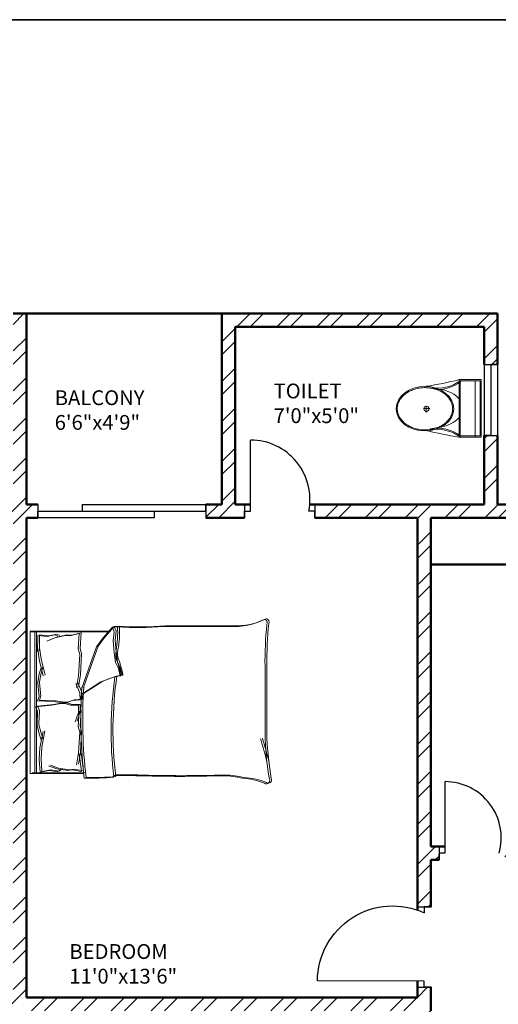
# Model space of a CAD drawing. Units: inches. Extents: x 963 to 2075, y 289 to 2657.
# Tile 95 of 98: x 1511 to 1672, y 2325 to 2657. Entities that reach past the tile are written whole.
import ezdxf

# ---------------------------------------------------------------- set-up
doc = ezdxf.new("R2010")
doc.units = ezdxf.units.IN
for name, color, linetype, lineweight in [('A-ANNO-TTLB', 7, 'Continuous', 35), ('A-AREA-IDEN', 7, 'Continuous', 18), ('A-DOOR', 4, 'Continuous', 25), ('A-FLOR-FIXT', 9, 'Continuous', 18), ('A-FURN', 8, 'Continuous', 18), ('A-GLAZ', 3, 'Continuous', 25), ('A-WALL', 7, 'Continuous', 50), ('A-WALL-PATT', 8, 'Continuous', 13)]:
    doc.layers.add(name, color=color, linetype=linetype, lineweight=lineweight)
doc.styles.get("Standard").update_dxf_attribs({"font": 'arial.ttf'})

# ---------------------------------------------------------------- blocks, each defined once
blk = doc.blocks.new('A$C31115884')
for p, q in [((283.1, 497.7), (223.4, 497.7)), ((257.5, 466.4), (257.5, 523.2)), ((0, 200), (0, 0)), ((520, 200), (0, 200)), ((10, 190), (10, 10)), ((510, 190), (10, 190)), ((510, 10), (510, 190)), ((520, 0), (520, 200)), ((510, 54.5), (0, 54.5)), ((10, 10), (510, 10)), ((0, 0), (520, 0))]:
    blk.add_line(p, q)
blk.add_circle((255.6, 496.4), 23.6)
for centre, radius, start, end in [((2777.7, -204.6), 2807, 165.4549, 171.71327), ((-294.5, 403.3), 364.7, 324.20913, 9.34987), ((-294.5, 403.3), 374.7, 324.20913, 9.34987), ((805.8, 403.3), 364.7, 170.65013, 215.79087), ((3237, 905), 2807, 188.28673, 194.5451), ((139.5, 406.2), 293.5, 315.84364, 2.65635), ((805.8, 403.3), 374.7, 179.20365, 215.79087), ((383.6, 406.2), 293.5, 190.27735, 224.15636)]:
    blk.add_arc(centre, radius, start, end)
blk.add_ellipse((256.2, 509.9), major_axis=(0, -260.7), ratio=0.772727)
blk.add_open_spline([(256.2, 259.2), (263.1, 259.2), (270, 259.7), (287.8, 262.3), (298.7, 265.1), (319.9, 273.1), (330.2, 278.4), (350.1, 291.1), (359.7, 298.7), (377.7, 315.9), (386.2, 325.5), (401.7, 346.6), (408.8, 358.1), (421.3, 382.5), (426.8, 395.5), (435.9, 422.4), (439.5, 436.4), (444.8, 465.1), (446.5, 479.7), (447.9, 509.2), (447.6, 524), (445, 553.3), (442.7, 567.8), (436.3, 596), (432.1, 609.7), (421.9, 636), (416, 648.6), (402.5, 672.1), (395, 683), (378.6, 703), (369.8, 712.1), (351.1, 728), (341.3, 734.8), (320.9, 746.2), (310.4, 750.7), (288.9, 757.3), (278, 759.4), (256, 761), (245, 760.6), (223.1, 757.2), (212.3, 754.3), (191.1, 746.1), (180.8, 740.7), (160.9, 727.8), (151.4, 720.1), (133.5, 702.7), (125.1, 693), (109.6, 671.7), (102.6, 660.2), (90.2, 635.7), (84.9, 622.7), (76, 595.6), (72.4, 581.6), (67.2, 552.9), (65.6, 538.2), (64.4, 508.8), (64.8, 494), (67.5, 464.7), (69.9, 450.2), (76.6, 422), (80.8, 408.3), (91.1, 382.2), (97.2, 369.7), (110.8, 346.3), (118.4, 335.4), (134.8, 315.6), (143.7, 306.7), (162.4, 290.9), (172.3, 284.2), (192.8, 273), (203.3, 268.6), (224.8, 262.2), (235.8, 260.2), (249.9, 259.3), (253, 259.2), (256.2, 259.2)], degree=3, knots=[0, 0, 0, 0, 0.110105, 0.110105, 0.285049, 0.285049, 0.459994, 0.459994, 0.634938, 0.634938, 0.809882, 0.809882, 0.984827, 0.984827, 1.159771, 1.159771, 1.334715, 1.334715, 1.50966, 1.50966, 1.684604, 1.684604, 1.859549, 1.859549, 2.034493, 2.034493, 2.209437, 2.209437, 2.384382, 2.384382, 2.559326, 2.559326, 2.73427, 2.73427, 2.909215, 2.909215, 3.084159, 3.084159, 3.259103, 3.259103, 3.434048, 3.434048, 3.608992, 3.608992, 3.783936, 3.783936, 3.958881, 3.958881, 4.133825, 4.133825, 4.30877, 4.30877, 4.483714, 4.483714, 4.658658, 4.658658, 4.833603, 4.833603, 5.008547, 5.008547, 5.183491, 5.183491, 5.358436, 5.358436, 5.53338, 5.53338, 5.708324, 5.708324, 5.883269, 5.883269, 6.058213, 6.058213, 6.233158, 6.233158, 6.283185, 6.283185, 6.283185, 6.283185])
blk = doc.blocks.new('BED-DOUBLE')
for p, q in [((1236.12, 2450.52), (1254.23, 2450.52)), ((1236.12, 2450.52), (1254.23, 2450.52)), ((1236.76, 2450.75), (1254.87, 2450.75)), ((1236.76, 2450.75), (1254.87, 2450.75)), ((1238.25, 2444.94), (1237.53, 2450.04)), ((1237.53, 2450.04), (1240.71, 2449.46)), ((1238.25, 2444.94), (1237.53, 2450.04)), ((1237.53, 2450.04), (1240.71, 2449.46)), ((1245.77, 2450.18), (1244.76, 2449.61)), ((1245.77, 2450.18), (1244.76, 2449.61)), ((1248.37, 2449.75), (1245.77, 2450.18)), ((1248.37, 2449.75), (1245.77, 2450.18)), ((1250.92, 2450.1), (1247.74, 2449.52)), ((1250.92, 2450.1), (1247.74, 2449.52)), ((1251.56, 2450.33), (1248.37, 2449.75)), ((1251.56, 2450.33), (1248.37, 2449.75)), ((1250.89, 2450.1), (1251.22, 2445.82)), ((1250.89, 2450.1), (1251.22, 2445.82)), ((1251.53, 2450.32), (1251.86, 2446.04)), ((1251.53, 2450.32), (1251.86, 2446.04)), ((1252.7, 2450.52), (1252.7, 2402.73)), ((1252.7, 2450.52), (1252.7, 2402.73)), ((1253.34, 2450.75), (1253.34, 2402.96)), ((1253.34, 2450.75), (1253.34, 2402.96)), ((1254.87, 2450.75), (1254.87, 2402.73)), ((1237.61, 2444.71), (1236.89, 2449.81)), ((1236.89, 2449.81), (1240.07, 2449.23)), ((1237.61, 2444.71), (1236.89, 2449.81)), ((1236.89, 2449.81), (1240.07, 2449.23)), ((1238.6, 2447.61), (1237.94, 2443.58)), ((1238.6, 2447.61), (1237.94, 2443.58)), ((1239.24, 2447.84), (1238.58, 2443.81)), ((1239.24, 2447.84), (1238.58, 2443.81)), ((1240.07, 2449.23), (1241.66, 2449.52)), ((1240.07, 2449.23), (1241.66, 2449.52)), ((1240.71, 2449.46), (1242.3, 2449.75)), ((1240.71, 2449.46), (1242.3, 2449.75)), ((1241.66, 2449.52), (1245.28, 2448.94)), ((1241.66, 2449.52), (1245.28, 2448.94)), ((1242.3, 2449.75), (1245.92, 2449.17)), ((1242.3, 2449.75), (1245.92, 2449.17)), ((1245.13, 2449.96), (1244.12, 2449.38)), ((1245.13, 2449.96), (1244.12, 2449.38)), ((1247.74, 2449.52), (1245.13, 2449.96)), ((1247.74, 2449.52), (1245.13, 2449.96)), ((1245.28, 2448.94), (1248.02, 2447.93)), ((1245.28, 2448.94), (1248.02, 2447.93)), ((1245.92, 2449.17), (1248.66, 2448.16)), ((1245.92, 2449.17), (1248.66, 2448.16)), ((1237.94, 2443.58), (1237.51, 2436.57)), ((1237.94, 2443.58), (1237.51, 2436.57)), ((1237.94, 2443.58), (1237.61, 2444.71)), ((1237.94, 2443.58), (1237.61, 2444.71)), ((1238.58, 2443.81), (1238.15, 2436.8)), ((1238.58, 2443.81), (1238.15, 2436.8)), ((1238.58, 2443.81), (1238.25, 2444.94)), ((1238.58, 2443.81), (1238.25, 2444.94)), ((1251.21, 2445.71), (1250.92, 2441.89)), ((1251.21, 2445.71), (1250.92, 2441.89)), ((1251.22, 2445.82), (1251.21, 2445.71)), ((1251.22, 2445.82), (1251.21, 2445.71)), ((1251.84, 2445.94), (1251.56, 2442.11)), ((1251.84, 2445.94), (1251.56, 2442.11)), ((1251.86, 2446.04), (1251.84, 2445.94)), ((1251.86, 2446.04), (1251.84, 2445.94)), ((1250.92, 2441.89), (1249.9, 2436.39)), ((1250.92, 2441.89), (1249.9, 2436.39)), ((1251.56, 2442.11), (1250.54, 2436.62)), ((1251.56, 2442.11), (1250.54, 2436.62)), ((1174.99, 2438.93), (1174.99, 2414.32)), ((1174.99, 2438.93), (1174.99, 2414.32)), ((1175.63, 2439.16), (1175.63, 2414.55)), ((1175.63, 2439.16), (1175.63, 2414.55)), ((1238.15, 2436.8), (1238.7, 2434.84)), ((1238.15, 2436.8), (1238.7, 2434.84)), ((1250.48, 2439.14), (1251.21, 2437.12)), ((1250.48, 2439.14), (1251.21, 2437.12)), ((1251.12, 2439.37), (1251.84, 2437.34)), ((1251.12, 2439.37), (1251.84, 2437.34)), ((1251.21, 2437.12), (1251.93, 2434.22)), ((1251.21, 2437.12), (1251.93, 2434.23)), ((1251.84, 2437.34), (1252.57, 2434.45)), ((1251.84, 2437.34), (1252.57, 2434.45)), ((1237.51, 2436.57), (1238.06, 2434.61)), ((1237.51, 2436.57), (1238.06, 2434.61)), ((1238.06, 2434.61), (1237.66, 2429.48)), ((1238.06, 2434.61), (1237.66, 2429.48)), ((1238.7, 2434.84), (1238.3, 2429.71)), ((1238.7, 2434.84), (1238.3, 2429.71)), ((1251.93, 2433.9), (1251.78, 2429.46)), ((1251.93, 2433.9), (1251.78, 2429.46)), ((1251.93, 2434.23), (1251.93, 2433.9)), ((1251.93, 2434.22), (1251.93, 2433.9)), ((1252.57, 2434.13), (1252.42, 2429.69)), ((1252.57, 2434.13), (1252.42, 2429.69)), ((1252.57, 2434.45), (1252.57, 2434.13)), ((1252.57, 2434.45), (1252.57, 2434.13)), ((1237.97, 2429.89), (1239.06, 2433.04)), ((1237.97, 2429.89), (1239.06, 2433.04)), ((1238.61, 2430.12), (1239.7, 2433.26)), ((1238.61, 2430.12), (1239.7, 2433.26)), ((1238.61, 2427.66), (1238.61, 2430.12)), ((1238.61, 2427.66), (1238.61, 2430.12)), ((1237.97, 2427.43), (1237.97, 2429.89)), ((1237.97, 2427.43), (1237.97, 2429.89)), ((1240.65, 2427.43), (1237.97, 2427.43)), ((1240.65, 2427.43), (1237.97, 2427.43)), ((1241.29, 2427.66), (1238.61, 2427.66)), ((1241.29, 2427.66), (1238.61, 2427.66)), ((1242.53, 2426.86), (1240.65, 2427.43)), ((1242.53, 2426.86), (1240.65, 2427.43)), ((1242.49, 2426.79), (1240.66, 2426.09)), ((1242.49, 2426.79), (1240.66, 2426.09)), ((1243.17, 2427.08), (1241.29, 2427.66)), ((1243.17, 2427.08), (1241.29, 2427.66)), ((1243.79, 2426.87), (1242.49, 2426.79)), ((1243.79, 2426.87), (1242.49, 2426.79)), ((1243.83, 2426.86), (1242.53, 2426.86)), ((1243.83, 2426.86), (1242.53, 2426.86)), ((1244.47, 2427.08), (1243.17, 2427.08)), ((1244.47, 2427.08), (1243.17, 2427.08)), ((1247, 2426.49), (1243.79, 2426.87)), ((1247, 2426.49), (1243.79, 2426.87)), ((1247.01, 2427.43), (1243.83, 2426.86)), ((1247.01, 2427.43), (1243.83, 2426.86)), ((1247.65, 2427.66), (1244.47, 2427.08)), ((1247.65, 2427.66), (1244.47, 2427.08)), ((1252.36, 2428.01), (1247.01, 2427.43)), ((1252.36, 2428.01), (1247.01, 2427.43)), ((1253, 2428.24), (1247.65, 2427.66)), ((1253, 2428.24), (1247.65, 2427.66)), ((1251.78, 2429.46), (1252.36, 2428.01)), ((1251.78, 2429.46), (1252.36, 2428.01)), ((1252.42, 2429.69), (1253, 2428.24)), ((1252.42, 2429.69), (1253, 2428.24)), ((1236.85, 2423.74), (1230.36, 2419.55)), ((1236.85, 2423.74), (1230.36, 2419.55)), ((1237.49, 2423.96), (1231, 2419.77)), ((1237.49, 2423.96), (1231, 2419.77)), ((1240.02, 2425.86), (1237.34, 2425.7)), ((1240.02, 2425.86), (1237.34, 2425.7)), ((1237.34, 2425.7), (1237.49, 2423.24)), ((1237.34, 2425.7), (1237.49, 2423.24)), ((1240.66, 2426.09), (1237.98, 2425.93)), ((1240.66, 2426.09), (1237.98, 2425.93)), ((1237.98, 2425.93), (1238.13, 2423.47)), ((1237.98, 2425.93), (1238.13, 2423.47)), ((1238.13, 2423.47), (1239.42, 2420.4)), ((1238.13, 2423.47), (1239.42, 2420.4)), ((1241.86, 2426.56), (1240.02, 2425.86)), ((1241.86, 2426.56), (1240.02, 2425.86)), ((1243.15, 2426.64), (1241.86, 2426.56)), ((1243.15, 2426.64), (1241.86, 2426.56)), ((1246.37, 2426.26), (1243.15, 2426.64)), ((1246.37, 2426.26), (1243.15, 2426.64)), ((1251.74, 2426.02), (1246.37, 2426.26)), ((1251.74, 2426.02), (1246.37, 2426.26)), ((1252.38, 2426.25), (1247, 2426.49)), ((1252.38, 2426.25), (1247, 2426.49)), ((1251.25, 2424.54), (1251.74, 2426.02)), ((1251.25, 2424.54), (1251.74, 2426.02)), ((1251.68, 2420.11), (1251.25, 2424.54)), ((1251.68, 2420.11), (1251.25, 2424.54)), ((1251.89, 2424.77), (1252.38, 2426.25)), ((1251.89, 2424.77), (1252.38, 2426.25)), ((1252.31, 2420.34), (1251.89, 2424.77)), ((1252.31, 2420.34), (1251.89, 2424.77)), ((1233.92, 2413.35), (1236.85, 2421.69)), ((1233.92, 2413.35), (1236.85, 2421.69)), ((1234.56, 2413.58), (1237.49, 2421.92)), ((1234.56, 2413.58), (1237.49, 2421.92)), ((1237.49, 2423.24), (1238.78, 2420.17)), ((1237.49, 2423.24), (1238.78, 2420.17)), ((1238.6, 2421.43), (1237.94, 2417.4)), ((1238.6, 2421.43), (1237.94, 2417.4)), ((1239.24, 2421.66), (1238.58, 2417.63)), ((1239.24, 2421.66), (1238.58, 2417.63)), ((1251.7, 2419.79), (1251.68, 2420.11)), ((1251.7, 2419.79), (1251.68, 2420.11)), ((1252.33, 2420.02), (1252.31, 2420.34)), ((1252.33, 2420.02), (1252.31, 2420.34)), ((1225.87, 2417.84), (1223.86, 2417.53)), ((1225.87, 2417.84), (1223.86, 2417.53)), ((1223.86, 2417.53), (1224.47, 2415.05)), ((1223.86, 2417.53), (1224.47, 2415.05)), ((1226.51, 2418.07), (1224.49, 2417.76)), ((1226.51, 2418.07), (1224.49, 2417.76)), ((1224.49, 2417.76), (1225.11, 2415.28)), ((1224.49, 2417.76), (1225.11, 2415.28)), ((1230.36, 2419.55), (1225.87, 2417.84)), ((1230.36, 2419.55), (1225.87, 2417.84)), ((1231, 2419.77), (1226.51, 2418.07)), ((1231, 2419.77), (1226.51, 2418.07)), ((1237.94, 2417.4), (1237.51, 2410.39)), ((1237.94, 2417.4), (1237.51, 2410.39)), ((1238.58, 2417.63), (1238.15, 2410.62)), ((1238.58, 2417.63), (1238.15, 2410.62)), ((1251.16, 2412.08), (1249.81, 2417.5)), ((1251.16, 2412.08), (1249.81, 2417.5)), ((1251.8, 2412.31), (1250.45, 2417.73)), ((1251.8, 2412.31), (1250.45, 2417.73)), ((1250.56, 2414.79), (1251.15, 2416.86)), ((1250.56, 2414.79), (1251.15, 2416.86)), ((1251.15, 2416.86), (1251.7, 2419.79)), ((1251.15, 2416.86), (1251.7, 2419.79)), ((1251.2, 2415.02), (1251.79, 2417.09)), ((1251.2, 2415.02), (1251.79, 2417.09)), ((1251.79, 2417.09), (1252.33, 2420.02)), ((1251.79, 2417.09), (1252.33, 2420.02)), ((1224.47, 2415.05), (1225.4, 2413.04)), ((1224.47, 2415.05), (1225.4, 2413.04)), ((1225.11, 2415.28), (1226.04, 2413.27)), ((1225.11, 2415.28), (1226.04, 2413.27)), ((1232.54, 2408), (1234.56, 2413.58)), ((1232.54, 2408), (1234.56, 2413.58)), ((1225.4, 2413.04), (1225.87, 2409.63)), ((1225.4, 2413.04), (1225.87, 2409.63)), ((1226.04, 2413.27), (1226.51, 2409.86)), ((1226.04, 2413.27), (1226.51, 2409.86)), ((1231.9, 2407.77), (1233.92, 2413.35)), ((1231.9, 2407.78), (1233.92, 2413.35)), ((1237.51, 2410.39), (1238.06, 2408.43)), ((1237.51, 2410.39), (1238.06, 2408.43)), ((1238.15, 2410.62), (1238.7, 2408.66)), ((1238.15, 2410.62), (1238.7, 2408.66)), ((1251.69, 2408.28), (1251.16, 2412.08)), ((1251.69, 2408.28), (1251.16, 2412.08)), ((1252.33, 2408.51), (1251.8, 2412.31)), ((1252.33, 2408.51), (1251.8, 2412.31)), ((1225.87, 2409.63), (1226.18, 2405.76)), ((1225.87, 2409.63), (1226.18, 2405.76)), ((1226.51, 2409.86), (1226.82, 2405.99)), ((1226.51, 2409.86), (1226.82, 2405.99)), ((1229.74, 2404.83), (1231.9, 2407.78)), ((1229.74, 2404.83), (1231.9, 2407.77)), ((1230.38, 2405.06), (1232.54, 2408)), ((1230.38, 2405.06), (1232.54, 2408)), ((1238.06, 2408.43), (1237.66, 2403.3)), ((1238.06, 2408.43), (1237.66, 2403.3)), ((1238.7, 2408.66), (1238.3, 2403.52)), ((1238.7, 2408.66), (1238.3, 2403.52)), ((1251.68, 2403.88), (1251.77, 2409.29)), ((1251.68, 2403.88), (1251.77, 2409.28)), ((1251.77, 2409.29), (1251.69, 2408.28)), ((1251.77, 2409.28), (1251.69, 2408.28)), ((1252.31, 2404.11), (1252.41, 2409.51)), ((1252.31, 2404.11), (1252.41, 2409.51)), ((1252.41, 2409.51), (1252.33, 2408.51)), ((1252.41, 2409.51), (1252.33, 2408.51)), ((1226.18, 2405.76), (1225.87, 2402.66)), ((1226.18, 2405.76), (1225.87, 2402.66)), ((1226.49, 2401.13), (1229.74, 2404.83)), ((1226.49, 2401.13), (1229.74, 2404.83)), ((1226.82, 2405.99), (1226.51, 2402.89)), ((1226.82, 2405.99), (1226.51, 2402.89)), ((1227.13, 2401.36), (1230.38, 2405.06)), ((1227.13, 2401.36), (1230.38, 2405.06)), ((1237.66, 2403.3), (1240.8, 2404.07)), ((1237.66, 2403.3), (1240.8, 2404.07)), ((1238.3, 2403.52), (1241.44, 2404.3)), ((1238.3, 2403.52), (1241.44, 2404.3)), ((1240.8, 2404.07), (1242.4, 2403.88)), ((1240.8, 2404.07), (1242.4, 2403.88)), ((1241.44, 2404.3), (1243.04, 2404.11)), ((1241.44, 2404.3), (1243.04, 2404.11)), ((1242.4, 2403.88), (1245.98, 2404.69)), ((1242.4, 2403.88), (1245.98, 2404.69)), ((1243.04, 2404.11), (1246.61, 2404.91)), ((1243.04, 2404.11), (1246.61, 2404.91)), ((1245.89, 2403.67), (1244.85, 2404.18)), ((1245.89, 2403.67), (1244.85, 2404.18)), ((1246.53, 2403.89), (1245.49, 2404.41)), ((1246.53, 2403.89), (1245.49, 2404.41)), ((1248.46, 2404.26), (1245.89, 2403.67)), ((1248.46, 2404.26), (1245.89, 2403.67)), ((1245.98, 2404.69), (1248.65, 2405.87)), ((1245.98, 2404.69), (1248.65, 2405.87)), ((1249.1, 2404.49), (1246.53, 2403.89)), ((1249.1, 2404.49), (1246.53, 2403.89)), ((1246.61, 2404.91), (1249.29, 2406.1)), ((1246.61, 2404.91), (1249.29, 2406.09)), ((1251.68, 2403.88), (1248.46, 2404.26)), ((1251.68, 2403.88), (1248.46, 2404.26)), ((1252.31, 2404.11), (1249.1, 2404.49)), ((1252.31, 2404.11), (1249.1, 2404.49)), ((1224.74, 2401.05), (1226.49, 2401.13, 3.87)), ((1224.74, 2401.05), (1226.49, 2401.13, 3.87)), ((1225.38, 2401.28), (1227.13, 2401.36, 3.87)), ((1225.38, 2401.28), (1227.13, 2401.36, 3.87)), ((1225.87, 2402.66), (1226.49, 2401.13)), ((1225.87, 2402.66), (1226.49, 2401.13)), ((1226.51, 2402.89), (1227.13, 2401.36)), ((1226.51, 2402.89), (1227.13, 2401.36)), ((1254.23, 2402.73), (1227.62, 2402.73)), ((1254.23, 2402.73), (1227.62, 2402.73)), ((1254.87, 2402.96), (1228.26, 2402.96)), ((1254.87, 2402.96), (1228.26, 2402.96)), ((1254.87, 2402.73), (1254.23, 2402.73))]:
    blk.add_line(p, q)
for centre, radius, start, end in [((1174.51, 2452.91), 1.09, 56.1736, 203.4781), ((1174.51, 2452.91), 1.09, 56.1736, 203.4781), ((1175.15, 2453.14), 1.09, 56.1736, 203.4781), ((1175.15, 2453.14), 1.09, 56.1736, 203.4781), ((1183.96, 2475.65), 23.56, 247.9751, 266.652), ((1183.96, 2475.65), 23.56, 247.9751, 266.652), ((1184.6, 2475.88), 23.56, 247.9751, 266.652), ((1184.6, 2475.88), 23.56, 247.9751, 266.652), ((1053.4, 2432.57), 121.76, 2.9958, 9.4091), ((1053.4, 2432.57), 121.76, 2.9958, 9.4091), ((1054.03, 2432.8), 121.76, 2.9958, 9.4091), ((1054.03, 2432.8), 121.76, 2.9958, 9.4091), ((1189.72, 2480.89), 29.63, 256.0648, 268.9113), ((1189.72, 2480.89), 29.63, 256.0648, 268.9113), ((1190.36, 2481.12), 29.63, 256.0648, 268.9113), ((1190.36, 2481.12), 29.63, 256.0648, 268.9113), ((1203.62, 1969.17), 482.31, 88.2277, 91.7185), ((1203.62, 1969.17), 482.31, 88.2277, 91.7185), ((1204.26, 1969.4), 482.31, 88.2277, 91.7185), ((1204.26, 1969.4), 482.31, 88.2277, 91.7185), ((1223.06, 2621.3), 170.11, 268.4762, 271.0082), ((1223.06, 2621.3), 170.11, 268.4762, 271.0082), ((1223.7, 2621.53), 170.11, 268.4762, 271.0082), ((1223.7, 2621.53), 170.11, 268.4762, 271.0082), ((1097.92, 2436.24), 129.02, 351.7845, 6.9006), ((1097.92, 2436.24), 129.02, 351.7845, 6.9006), ((1234.14, 2368.83), 83.31, 88.7218, 95.604), ((1234.14, 2368.83), 83.31, 88.7218, 95.604), ((1098.56, 2436.47), 129.02, 351.7845, 6.9006), ((1098.56, 2436.47), 129.02, 351.7845, 6.9006), ((1234.78, 2369.06), 83.31, 88.7218, 95.604), ((1234.78, 2369.06), 83.31, 88.7218, 95.604), ((1072.18, 2432.64), 164.97, 356.0865, 6.7821), ((1072.18, 2432.64), 164.97, 356.0865, 6.7821), ((1072.82, 2432.86), 164.97, 356.0865, 6.7821), ((1072.82, 2432.86), 164.97, 356.0865, 6.7821), ((1278.58, 2471.44), 106.46, 193.3832, 197.7053), ((1278.58, 2471.44), 106.46, 193.3832, 197.7053), ((1277.94, 2471.22), 106.46, 193.3832, 197.7053), ((1277.94, 2471.22), 106.46, 193.3832, 197.7053), ((1223.79, 2417.36), 0.185, 70.2464, 181.1377), ((1223.79, 2417.36), 0.185, 70.2464, 181.1377), ((1252.75, 2422.84), 29.65, 190.6617, 199.8806), ((1252.75, 2422.84), 29.65, 190.6617, 199.8806), ((1224.43, 2417.59), 0.185, 70.2464, 181.1377), ((1224.43, 2417.59), 0.185, 70.2464, 181.1377), ((1253.39, 2423.07), 29.65, 190.6617, 199.8806), ((1253.39, 2423.07), 29.65, 190.6617, 199.8806), ((1041.96, 2412.84), 133.04, 354.4998, 0.6351), ((1041.96, 2412.84), 133.04, 354.4998, 0.6351), ((1042.6, 2413.07), 133.04, 354.4998, 0.6351), ((1042.6, 2413.07), 133.04, 354.4998, 0.6351), ((1219.17, 2410.25), 6.22, 348.6608, 23.7384), ((1219.17, 2410.25), 6.22, 348.6608, 23.7384), ((1219.81, 2410.48), 6.22, 348.6608, 23.7384), ((1219.81, 2410.48), 6.22, 348.6608, 23.7384), ((1260.89, 2402.67), 36.18, 169.8763, 182.5657), ((1260.89, 2402.67), 36.18, 169.8763, 182.5657), ((1261.53, 2402.9), 36.18, 169.8763, 182.5657), ((1261.53, 2402.9), 36.18, 169.8763, 182.5657), ((1176, 2399.81), 1.1, 152.6588, 266.02), ((1176, 2399.81), 1.1, 152.6588, 266.02), ((1185.57, 2377.84), 23.07, 87.4714, 116.4681), ((1185.57, 2377.84), 23.07, 87.4714, 116.4681), ((1186.21, 2378.07), 23.07, 87.4714, 116.4681), ((1186.21, 2378.07), 23.07, 87.4714, 116.4681), ((1186.41, 6962.74), 4561.86, 270.00217, 270.28689), ((1186.41, 6962.74), 4561.86, 270.00217, 270.28689), ((1187.05, 6962.97), 4561.86, 270.00217, 270.28689), ((1187.05, 6962.97), 4561.86, 270.00217, 270.28689), ((1217.92, 2271.73), 129.5, 86.9791, 93.8365), ((1217.92, 2271.73), 129.5, 86.9791, 93.8365), ((1218.56, 2271.96), 129.5, 86.9791, 93.8365), ((1218.56, 2271.96), 129.5, 86.9791, 93.8365), ((1175.36, 2399.58), 1.1, 152.6588, 266.02), ((1175.36, 2399.58), 1.1, 152.6588, 266.02)]:
    blk.add_arc(centre, radius, start, end)
blk = doc.blocks.new('DOOR-1')
for p, q in [((25.38, 2.25), (25.38, 38.25)), ((0.32, 4.5), (0.32, 0)), ((27.38, 4.5), (27.38, 0)), ((0.32, 0), (0.32, 2.25)), ((0.32, 2.25), (2.32, 2.25)), ((27.38, 2.25), (25.38, 2.25)), ((27.38, 0), (27.38, 2.25))]:
    blk.add_line(p, q)
blk.add_arc((25.38, 12.86), 25.39, 90, 204.7158)

msp = doc.modelspace()

# ---------------------------------------------------------------- hatches: boundary and pattern name
at = {"layer": 'A-WALL-PATT'}
h = msp.add_hatch(dxfattribs=at)
h.set_pattern_fill('ANSI32', color=256)
h.paths.add_polyline_path([(1296.92, 2558.32), (1203.92, 2558.32), (1203.92, 2493.82), (1191.53, 2493.82), (1191.53, 2489.32), (1211.06, 2489.32), (1211.06, 2492.02), (1211.06, 2493.82), (1208.42, 2493.82), (1208.42, 2553.82), (1292.42, 2553.82), (1292.42, 2538.86), (1296.92, 2538.86)])
h.paths.add_polyline_path([(1442.42, 2558.32), (1349.42, 2558.32), (1349.42, 2538.94), (1353.92, 2538.94), (1353.92, 2553.82), (1437.92, 2553.82), (1437.92, 2493.82), (1434.54, 2493.82), (1434.54, 2489.32), (1448.31, 2489.32), (1448.31, 2491.57), (1448.31, 2493.82), (1442.42, 2493.82)])
h.paths.add_polyline_path([(1415.55, 2491.57), (1415.55, 2493.82), (1340.94, 2493.82), (1340.94, 2489.32), (1371.92, 2489.32), (1371.92, 2378.32), (1367.6, 2378.32), (1367.6, 2373.82), (1371.92, 2373.82), (1371.92, 2355.19), (1376.42, 2355.19), (1376.42, 2489.32), (1415.55, 2489.32)])
h.paths.add_polyline_path([(1304.94, 2491.57), (1304.94, 2493.82), (1296.92, 2493.82), (1296.92, 2514.86), (1292.42, 2514.86), (1292.42, 2493.82), (1232.81, 2493.82), (1232.81, 2489.32), (1256.42, 2489.32), (1256.42, 2327.32), (1253.71, 2327.32), (1253.71, 2322.82), (1328.42, 2322.82), (1328.42, 2331.15), (1323.92, 2331.15), (1323.92, 2327.32), (1260.92, 2327.32), (1260.92, 2373.82), (1323.92, 2373.82), (1323.92, 2357.81), (1328.42, 2357.81), (1328.42, 2373.82), (1346.01, 2373.82), (1346.01, 2376.07), (1346.01, 2378.32), (1260.92, 2378.32), (1260.92, 2489.32), (1304.94, 2489.32)])
h.paths.add_polyline_path([(1226.65, 2327.32), (1124.42, 2327.32), (1124.42, 2347.45), (1119.92, 2347.45), (1119.92, 2322.82), (1163.42, 2322.82), (1163.42, 2305.43), (1165.67, 2305.43), (1167.92, 2305.43), (1167.92, 2322.82), (1226.65, 2322.82), (1226.65, 2325.07)])
h.paths.add_polyline_path([(1095.92, 2489.32), (1124.42, 2489.32), (1131.53, 2489.32), (1131.53, 2491.57), (1131.53, 2493.82), (1119.92, 2493.82), (1091.42, 2493.82), (1091.42, 2417.32), (1095.92, 2417.32), (1119.92, 2417.32), (1119.92, 2407.45), (1124.42, 2407.45), (1124.42, 2421.82), (1095.92, 2421.82)])
h.paths.add_polyline_path([(1512.92, 2558.32), (1508.42, 2558.32), (1508.42, 2493.82), (1503.4, 2493.82), (1503.4, 2489.32), (1508.42, 2489.32), (1508.42, 2327.32), (1376.42, 2327.32), (1376.42, 2330.27), (1371.92, 2330.27), (1371.92, 2298.74), (1376.42, 2298.74), (1376.42, 2322.82), (1508.42, 2322.82), (1508.42, 2165.32), (1504.26, 2165.32), (1504.26, 2160.82), (1508.42, 2160.82), (1508.42, 2108.32), (1512.92, 2108.32), (1512.92, 2160.82), (1516.18, 2160.82), (1516.18, 2163.07), (1516.18, 2165.32), (1512.92, 2165.32), (1512.92, 2322.82), (1644.92, 2322.82), (1644.92, 2298.74), (1649.42, 2298.74), (1649.42, 2322.82), (1649.42, 2330.94), (1647.17, 2330.94), (1644.92, 2330.94), (1644.92, 2327.32), (1512.92, 2327.32), (1512.92, 2489.32), (1516.76, 2489.32), (1516.76, 2491.57), (1516.76, 2493.82), (1512.92, 2493.82)])
h.paths.add_polyline_path([(1671.92, 2558.32), (1578.92, 2558.32), (1578.92, 2493.82), (1573.53, 2493.82), (1573.53, 2489.32), (1586.54, 2489.32), (1586.54, 2491.57), (1586.54, 2493.82), (1583.42, 2493.82), (1583.42, 2553.82), (1667.42, 2553.82), (1667.42, 2541.11), (1671.92, 2541.11)])
h.paths.add_polyline_path([(1681.26, 2493.82), (1671.92, 2493.82), (1671.92, 2517.11), (1667.42, 2517.11), (1667.42, 2493.82), (1610.22, 2493.82), (1610.22, 2489.32), (1644.92, 2489.32), (1644.92, 2357.87), (1649.42, 2357.87), (1649.42, 2373.82), (1652.2, 2373.82), (1652.2, 2375.83), (1652.2, 2378.32), (1649.42, 2378.32), (1649.42, 2489.32), (1681.26, 2489.32), (1681.26, 2491.57)])
h.paths.add_polyline_path([(1821.92, 2558.32), (1728.92, 2558.32), (1728.92, 2541), (1733.42, 2541), (1733.42, 2553.82), (1817.42, 2553.82), (1817.42, 2493.82), (1813.51, 2493.82), (1813.51, 2489.32), (1830.08, 2489.32), (1830.08, 2491.57), (1830.08, 2493.82), (1821.92, 2493.82)])
h.paths.add_polyline_path([(1794.24, 2493.82), (1717.26, 2493.82), (1717.26, 2489.32), (1760.42, 2489.32), (1760.42, 2378.32), (1674.4, 2378.32), (1674.4, 2373.82), (1692.92, 2373.82), (1692.92, 2356.95), (1697.42, 2356.95), (1697.42, 2373.82), (1760.42, 2373.82), (1760.42, 2327.32), (1697.42, 2327.32), (1697.42, 2333.34), (1692.92, 2333.34), (1692.92, 2322.82), (1768.04, 2322.82), (1768.04, 2325.07), (1768.04, 2327.32), (1764.92, 2327.32), (1764.92, 2489.32), (1794.24, 2489.32)])
h.paths.add_polyline_path([(1733.42, 2517), (1728.92, 2517), (1728.92, 2493.82), (1733.42, 2493.82)], flags=17)
h.paths.add_polyline_path([(1929.92, 2493.82), (1890.08, 2493.82), (1890.08, 2489.32), (1896.92, 2489.32), (1925.42, 2489.32), (1925.42, 2421.82), (1896.92, 2421.82), (1896.92, 2408.32), (1901.42, 2408.32), (1901.42, 2417.32), (1925.42, 2417.32), (1929.92, 2417.32)])
h.paths.add_polyline_path([(1901.42, 2348.32), (1896.92, 2348.32), (1896.92, 2327.32), (1800.42, 2327.32), (1800.42, 2322.82), (1853.42, 2322.82), (1853.42, 2309.45), (1857.92, 2309.45), (1857.92, 2322.82), (1901.42, 2322.82)])
h.paths.add_polyline_path([(1857.92, 2249.45), (1853.42, 2249.45), (1853.42, 2214.82), (1686.31, 2214.82), (1686.31, 2210.32), (1853.42, 2210.32), (1853.42, 2202.13), (1857.92, 2202.13), (1857.92, 2210.32)])
h.paths.add_polyline_path([(1857.92, 2142.13), (1853.42, 2142.13), (1853.42, 2115.42), (1841.42, 2115.42), (1841.42, 2088.53), (1841.42, 2046.95), (1845.92, 2046.95), (1845.92, 2110.92), (1905.92, 2110.92), (1905.92, 2092.52), (1910.42, 2092.52), (1910.42, 2115.42), (1857.92, 2115.42)])
h.paths.add_polyline_path([(1532.44, 1482.34), (1573.46, 1482.34), (1573.46, 1501), (1532.44, 1501)], flags=9)
h.paths.add_polyline_path([(1438.66, 1486.3), (1479.68, 1486.3), (1479.68, 1504.96), (1438.66, 1504.96)], flags=9)
h.paths.add_polyline_path([(1411.22, 1365.31), (1659.14, 1365.31), (1659.14, 1402.4), (1411.22, 1402.4)], flags=9)
h.paths.add_polyline_path([(1185.67, 2296.3), (1248.16, 2296.3), (1248.16, 2314.95), (1185.67, 2314.95)], flags=9)
h.paths.add_polyline_path([(1177.31, 2187.35), (1216.15, 2187.35), (1216.15, 2206.01), (1177.31, 2206.01)], flags=9)
h.paths.add_polyline_path([(1295.1, 1602.08), (1328.26, 1602.08), (1328.26, 1620.74), (1295.1, 1620.74)], flags=9)
h.paths.add_polyline_path([(1525.13, 2005.99), (1558.39, 2005.99), (1558.39, 2024.65), (1525.13, 2024.65)], flags=9)
h.paths.add_polyline_path([(1459.61, 1977.13), (1472.19, 1977.13), (1472.19, 1987.43), (1459.61, 1987.43)], flags=9)
h.paths.add_polyline_path([(1467.81, 2053.68), (1480.02, 2053.68), (1480.02, 2063.98), (1467.81, 2063.98)], flags=9)
h.paths.add_polyline_path([(1555.18, 2119.02), (1584.56, 2119.02), (1584.56, 2137.68), (1555.18, 2137.68)], flags=25)
h.paths.add_polyline_path([(1405.39, 2115.29), (1444.48, 2115.29), (1444.48, 2133.95), (1405.39, 2133.95)], flags=25)
h.paths.add_polyline_path([(1698.48, 2004.26), (1727.69, 2004.26), (1727.69, 2022.92), (1698.48, 2022.92)], flags=9)
h.paths.add_polyline_path([(1612.16, 1972.86), (1629.02, 1972.86), (1629.02, 1983.16), (1612.16, 1983.16)], flags=9)
h.paths.add_polyline_path([(1608.29, 2060.04), (1625.15, 2060.04), (1625.15, 2070.34), (1608.29, 2070.34)], flags=9)
h.paths.add_polyline_path([(1527.95, 1684.4), (1566.79, 1684.4), (1566.79, 1703.06), (1527.95, 1703.06)], flags=9)
h.paths.add_polyline_path([(1422.79, 1683.59), (1461.63, 1683.59), (1461.63, 1702.25), (1422.79, 1702.25)], flags=9)
h.paths.add_polyline_path([(1531.26, 1732.46), (1574.01, 1732.46), (1574.01, 1751.12), (1531.26, 1751.12)], flags=9)
h.paths.add_polyline_path([(1402.87, 1732.85), (1439.8, 1732.85), (1439.8, 1751.5), (1402.87, 1751.5)], flags=9)
h.paths.add_polyline_path([(1243.12, 1923.13), (1281.96, 1923.13), (1281.96, 1941.79), (1243.12, 1941.79)], flags=9)
h.paths.add_polyline_path([(1181.75, 1792.27), (1244.24, 1792.27), (1244.24, 1810.93), (1181.75, 1810.93)], flags=9)
h.paths.add_polyline_path([(1265.82, 1670.3), (1316.07, 1670.3), (1316.07, 1688.96), (1265.82, 1688.96)], flags=9)
h.paths.add_polyline_path([(1140.26, 1676.05), (1179.1, 1676.05), (1179.1, 1694.71), (1140.26, 1694.71)], flags=9)
h.paths.add_polyline_path([(1107.49, 1490.89), (1143.37, 1490.89), (1143.37, 1509.55), (1107.49, 1509.55)], flags=9)
h.paths.add_polyline_path([(1217.58, 1483.9), (1246.74, 1483.9), (1246.74, 1502.56), (1217.58, 1502.56)], flags=9)
h.paths.add_polyline_path([(1389.21, 1486.92), (1418.37, 1486.92), (1418.37, 1505.58), (1389.21, 1505.58)], flags=9)
h.paths.add_polyline_path([(1672.21, 1602.08), (1705.37, 1602.08), (1705.37, 1620.74), (1672.21, 1620.74)], flags=9)
h.paths.add_polyline_path([(1752.08, 1522.64), (1781.24, 1522.64), (1781.24, 1541.3), (1752.08, 1541.3)], flags=9)
h.paths.add_polyline_path([(1848.27, 1491.26), (1884.16, 1491.26), (1884.16, 1509.92), (1848.27, 1509.92)], flags=9)
h.paths.add_polyline_path([(1822.47, 1685.62), (1861.31, 1685.62), (1861.31, 1704.28), (1822.47, 1704.28)], flags=9)
h.paths.add_polyline_path([(1713.19, 1672.23), (1763.44, 1672.23), (1763.44, 1690.89), (1713.19, 1690.89)], flags=9)
h.paths.add_polyline_path([(1736.62, 1790.58), (1799.11, 1790.58), (1799.11, 1809.24), (1736.62, 1809.24)], flags=9)
h.paths.add_polyline_path([(1691.49, 1916.36), (1730.33, 1916.36), (1730.33, 1935.01), (1691.49, 1935.01)], flags=9)
h.paths.add_polyline_path([(1764.87, 1973.92), (1794.31, 1973.92), (1794.31, 1992.58), (1764.87, 1992.58)], flags=9)
h.paths.add_polyline_path([(1767.85, 2034.02), (1797.29, 2034.02), (1797.29, 2052.67), (1767.85, 2052.67)], flags=9)
h.paths.add_polyline_path([(1851.59, 2060.33), (1880.75, 2060.33), (1880.75, 2078.99), (1851.59, 2078.99)], flags=25)
h.paths.add_polyline_path([(1688.49, 2086.87), (1727.33, 2086.87), (1727.33, 2105.53), (1688.49, 2105.53)], flags=9)
h.paths.add_polyline_path([(1537.74, 2293.58), (1580.49, 2293.58), (1580.49, 2312.24), (1537.74, 2312.24)], flags=25)
h.paths.add_polyline_path([(1425.59, 2296.11), (1468.34, 2296.11), (1468.34, 2314.77), (1425.59, 2314.77)], flags=25)
h.paths.add_polyline_path([(1278.52, 2004.18), (1307.72, 2004.18), (1307.72, 2022.84), (1278.52, 2022.84)], flags=9)
h.paths.add_polyline_path([(1193.28, 1973.63), (1222.72, 1973.63), (1222.72, 1992.29), (1193.28, 1992.29)], flags=9)
h.paths.add_polyline_path([(1192.41, 2040.58), (1221.84, 2040.58), (1221.84, 2059.23), (1192.41, 2059.23)], flags=9)
h.paths.add_polyline_path([(1130.6, 1951.39), (1159.76, 1951.39), (1159.76, 1970.05), (1130.6, 1970.05)], flags=9)
h.paths.add_polyline_path([(1132.83, 2052.49), (1161.98, 2052.49), (1161.98, 2071.15), (1132.83, 2071.15)], flags=9)
h.paths.add_polyline_path([(1265.13, 2334.62), (1315.38, 2334.62), (1315.38, 2353.28), (1265.13, 2353.28)], flags=25)
h.paths.add_polyline_path([(1136.74, 2330.79), (1175.58, 2330.79), (1175.58, 2349.44), (1136.74, 2349.44)], flags=9)
h.paths.add_polyline_path([(1287.42, 2417.2), (1320.58, 2417.2), (1320.58, 2435.86), (1287.42, 2435.86)], flags=25)
h.paths.add_polyline_path([(1430.99, 2329.16), (1469.83, 2329.16), (1469.83, 2347.82), (1430.99, 2347.82)], flags=25)
h.paths.add_polyline_path([(1525.42, 2329.21), (1564.26, 2329.21), (1564.26, 2347.87), (1525.42, 2347.87)], flags=25)
h.paths.add_polyline_path([(1684.52, 2382.8), (1717.68, 2382.8), (1717.68, 2401.46), (1684.52, 2401.46)], flags=25)
h.paths.add_polyline_path([(1704.81, 2340.29), (1755.05, 2340.29), (1755.05, 2358.95), (1704.81, 2358.95)], flags=25)
h.paths.add_polyline_path([(1694.11, 2287.76), (1756.6, 2287.76), (1756.6, 2306.41), (1694.11, 2306.41)], flags=9)
h.paths.add_polyline_path([(1815.78, 2329.86), (1854.62, 2329.86), (1854.62, 2348.52), (1815.78, 2348.52)], flags=9)
h.paths.add_polyline_path([(1842.87, 2514.26), (1878.76, 2514.26), (1878.76, 2532.91), (1842.87, 2532.91)], flags=9)
h.paths.add_polyline_path([(1769.51, 2531.45), (1798.67, 2531.45), (1798.67, 2550.1), (1769.51, 2550.1)], flags=25)
h.paths.add_polyline_path([(1594.77, 2518.47), (1623.93, 2518.47), (1623.93, 2537.13), (1594.77, 2537.13)], flags=25)
h.paths.add_polyline_path([(1520.72, 2516.18), (1556.61, 2516.18), (1556.61, 2534.84), (1520.72, 2534.84)], flags=25)
h.paths.add_polyline_path([(1464.46, 2516.69), (1500.34, 2516.69), (1500.34, 2535.35), (1464.46, 2535.35)], flags=25)
h.paths.add_polyline_path([(1365.7, 2528.97), (1394.85, 2528.97), (1394.85, 2547.63), (1365.7, 2547.63)], flags=25)
h.paths.add_polyline_path([(1222.84, 2516.23), (1252, 2516.23), (1252, 2534.89), (1222.84, 2534.89)], flags=25)
h.paths.add_polyline_path([(1104.55, 2509.6), (1140.43, 2509.6), (1140.43, 2528.26), (1104.55, 2528.26)], flags=9)
h = msp.add_hatch(dxfattribs=at)
h.set_pattern_fill('ANSI32', color=256)
h.paths.add_polyline_path([(1335.97, 2212.57), (1335.97, 2214.82), (1167.92, 2214.82), (1167.92, 2245.43), (1163.42, 2245.43), (1163.42, 2210.32), (1163.42, 2194.81), (1167.92, 2194.81), (1167.92, 2210.32), (1335.97, 2210.32)])
h.paths.add_polyline_path([(1532.44, 1482.34), (1573.46, 1482.34), (1573.46, 1501), (1532.44, 1501)], flags=9)
h.paths.add_polyline_path([(1438.66, 1486.3), (1479.68, 1486.3), (1479.68, 1504.96), (1438.66, 1504.96)], flags=9)
h.paths.add_polyline_path([(1411.22, 1365.31), (1659.14, 1365.31), (1659.14, 1402.4), (1411.22, 1402.4)], flags=9)
h.paths.add_polyline_path([(1185.67, 2296.3), (1248.16, 2296.3), (1248.16, 2314.95), (1185.67, 2314.95)], flags=9)
h.paths.add_polyline_path([(1177.31, 2187.35), (1216.15, 2187.35), (1216.15, 2206.01), (1177.31, 2206.01)], flags=9)
h.paths.add_polyline_path([(1295.1, 1602.08), (1328.26, 1602.08), (1328.26, 1620.74), (1295.1, 1620.74)], flags=9)
h.paths.add_polyline_path([(1525.13, 2005.99), (1558.39, 2005.99), (1558.39, 2024.65), (1525.13, 2024.65)], flags=9)
h.paths.add_polyline_path([(1459.61, 1977.13), (1472.19, 1977.13), (1472.19, 1987.43), (1459.61, 1987.43)], flags=9)
h.paths.add_polyline_path([(1467.81, 2053.68), (1480.02, 2053.68), (1480.02, 2063.98), (1467.81, 2063.98)], flags=9)
h.paths.add_polyline_path([(1555.18, 2119.02), (1584.56, 2119.02), (1584.56, 2137.68), (1555.18, 2137.68)], flags=9)
h.paths.add_polyline_path([(1405.39, 2115.29), (1444.48, 2115.29), (1444.48, 2133.95), (1405.39, 2133.95)], flags=9)
h.paths.add_polyline_path([(1698.48, 2004.26), (1727.69, 2004.26), (1727.69, 2022.92), (1698.48, 2022.92)], flags=9)
h.paths.add_polyline_path([(1612.16, 1972.86), (1629.02, 1972.86), (1629.02, 1983.16), (1612.16, 1983.16)], flags=9)
h.paths.add_polyline_path([(1608.29, 2060.04), (1625.15, 2060.04), (1625.15, 2070.34), (1608.29, 2070.34)], flags=9)
h.paths.add_polyline_path([(1527.95, 1684.4), (1566.79, 1684.4), (1566.79, 1703.06), (1527.95, 1703.06)], flags=9)
h.paths.add_polyline_path([(1422.79, 1683.59), (1461.63, 1683.59), (1461.63, 1702.25), (1422.79, 1702.25)], flags=9)
h.paths.add_polyline_path([(1531.26, 1732.46), (1574.01, 1732.46), (1574.01, 1751.12), (1531.26, 1751.12)], flags=9)
h.paths.add_polyline_path([(1402.87, 1732.85), (1439.8, 1732.85), (1439.8, 1751.5), (1402.87, 1751.5)], flags=9)
h.paths.add_polyline_path([(1243.12, 1923.13), (1281.96, 1923.13), (1281.96, 1941.79), (1243.12, 1941.79)], flags=9)
h.paths.add_polyline_path([(1181.75, 1792.27), (1244.24, 1792.27), (1244.24, 1810.93), (1181.75, 1810.93)], flags=9)
h.paths.add_polyline_path([(1265.82, 1670.3), (1316.07, 1670.3), (1316.07, 1688.96), (1265.82, 1688.96)], flags=9)
h.paths.add_polyline_path([(1140.26, 1676.05), (1179.1, 1676.05), (1179.1, 1694.71), (1140.26, 1694.71)], flags=9)
h.paths.add_polyline_path([(1107.49, 1490.89), (1143.37, 1490.89), (1143.37, 1509.55), (1107.49, 1509.55)], flags=9)
h.paths.add_polyline_path([(1217.58, 1483.9), (1246.74, 1483.9), (1246.74, 1502.56), (1217.58, 1502.56)], flags=9)
h.paths.add_polyline_path([(1389.21, 1486.92), (1418.37, 1486.92), (1418.37, 1505.58), (1389.21, 1505.58)], flags=9)
h.paths.add_polyline_path([(1672.21, 1602.08), (1705.37, 1602.08), (1705.37, 1620.74), (1672.21, 1620.74)], flags=9)
h.paths.add_polyline_path([(1752.08, 1522.64), (1781.24, 1522.64), (1781.24, 1541.3), (1752.08, 1541.3)], flags=9)
h.paths.add_polyline_path([(1848.27, 1491.26), (1884.16, 1491.26), (1884.16, 1509.92), (1848.27, 1509.92)], flags=9)
h.paths.add_polyline_path([(1822.47, 1685.62), (1861.31, 1685.62), (1861.31, 1704.28), (1822.47, 1704.28)], flags=9)
h.paths.add_polyline_path([(1713.19, 1672.23), (1763.44, 1672.23), (1763.44, 1690.89), (1713.19, 1690.89)], flags=9)
h.paths.add_polyline_path([(1736.62, 1790.58), (1799.11, 1790.58), (1799.11, 1809.24), (1736.62, 1809.24)], flags=9)
h.paths.add_polyline_path([(1691.49, 1916.36), (1730.33, 1916.36), (1730.33, 1935.01), (1691.49, 1935.01)], flags=9)
h.paths.add_polyline_path([(1764.87, 1973.92), (1794.31, 1973.92), (1794.31, 1992.58), (1764.87, 1992.58)], flags=9)
h.paths.add_polyline_path([(1767.85, 2034.02), (1797.29, 2034.02), (1797.29, 2052.67), (1767.85, 2052.67)], flags=9)
h.paths.add_polyline_path([(1851.59, 2060.33), (1880.75, 2060.33), (1880.75, 2078.99), (1851.59, 2078.99)], flags=9)
h.paths.add_polyline_path([(1688.49, 2086.87), (1727.33, 2086.87), (1727.33, 2105.53), (1688.49, 2105.53)], flags=9)
h.paths.add_polyline_path([(1537.74, 2293.58), (1580.49, 2293.58), (1580.49, 2312.24), (1537.74, 2312.24)], flags=9)
h.paths.add_polyline_path([(1425.59, 2296.11), (1468.34, 2296.11), (1468.34, 2314.77), (1425.59, 2314.77)], flags=9)
h.paths.add_polyline_path([(1278.52, 2004.18), (1307.72, 2004.18), (1307.72, 2022.84), (1278.52, 2022.84)], flags=9)
h.paths.add_polyline_path([(1193.28, 1973.63), (1222.72, 1973.63), (1222.72, 1992.29), (1193.28, 1992.29)], flags=9)
h.paths.add_polyline_path([(1192.41, 2040.58), (1221.84, 2040.58), (1221.84, 2059.23), (1192.41, 2059.23)], flags=9)
h.paths.add_polyline_path([(1130.6, 1951.39), (1159.76, 1951.39), (1159.76, 1970.05), (1130.6, 1970.05)], flags=9)
h.paths.add_polyline_path([(1132.83, 2052.49), (1161.98, 2052.49), (1161.98, 2071.15), (1132.83, 2071.15)], flags=9)
h.paths.add_polyline_path([(1265.13, 2334.62), (1315.38, 2334.62), (1315.38, 2353.28), (1265.13, 2353.28)], flags=9)
h.paths.add_polyline_path([(1136.74, 2330.79), (1175.58, 2330.79), (1175.58, 2349.44), (1136.74, 2349.44)], flags=9)
h.paths.add_polyline_path([(1287.42, 2417.2), (1320.58, 2417.2), (1320.58, 2435.86), (1287.42, 2435.86)], flags=9)
h.paths.add_polyline_path([(1430.99, 2329.16), (1469.83, 2329.16), (1469.83, 2347.82), (1430.99, 2347.82)], flags=9)
h.paths.add_polyline_path([(1525.42, 2329.21), (1564.26, 2329.21), (1564.26, 2347.87), (1525.42, 2347.87)], flags=9)
h.paths.add_polyline_path([(1684.52, 2382.8), (1717.68, 2382.8), (1717.68, 2401.46), (1684.52, 2401.46)], flags=9)
h.paths.add_polyline_path([(1704.81, 2340.29), (1755.05, 2340.29), (1755.05, 2358.95), (1704.81, 2358.95)], flags=9)
h.paths.add_polyline_path([(1694.11, 2287.76), (1756.6, 2287.76), (1756.6, 2306.41), (1694.11, 2306.41)], flags=9)
h.paths.add_polyline_path([(1815.78, 2329.86), (1854.62, 2329.86), (1854.62, 2348.52), (1815.78, 2348.52)], flags=9)
h.paths.add_polyline_path([(1842.87, 2514.26), (1878.76, 2514.26), (1878.76, 2532.91), (1842.87, 2532.91)], flags=9)
h.paths.add_polyline_path([(1769.51, 2531.45), (1798.67, 2531.45), (1798.67, 2550.1), (1769.51, 2550.1)], flags=9)
h.paths.add_polyline_path([(1594.77, 2518.47), (1623.93, 2518.47), (1623.93, 2537.13), (1594.77, 2537.13)], flags=9)
h.paths.add_polyline_path([(1520.72, 2516.18), (1556.61, 2516.18), (1556.61, 2534.84), (1520.72, 2534.84)], flags=9)
h.paths.add_polyline_path([(1464.46, 2516.69), (1500.34, 2516.69), (1500.34, 2535.35), (1464.46, 2535.35)], flags=9)
h.paths.add_polyline_path([(1365.7, 2528.97), (1394.85, 2528.97), (1394.85, 2547.63), (1365.7, 2547.63)], flags=9)
h.paths.add_polyline_path([(1222.84, 2516.23), (1252, 2516.23), (1252, 2534.89), (1222.84, 2534.89)], flags=9)
h.paths.add_polyline_path([(1104.55, 2509.6), (1140.43, 2509.6), (1140.43, 2528.26), (1104.55, 2528.26)], flags=9)

# ---------------------------------------------------------------- linework, layer by layer
at = {"layer": 'A-ANNO-TTLB'}
msp.add_lwpolyline([(962.81, 2657.49), (2074.6, 2657.49), (2074.6, 1303.08), (962.81, 1303.08)], close=True, dxfattribs=at)
at = {"layer": 'A-DOOR'}
for p, q in [((1588.54, 2491.57), (1588.54, 2515.57)), ((1586.54, 2493.82), (1586.54, 2489.32)), ((1610.22, 2493.82), (1610.22, 2489.32)), ((1586.54, 2489.32), (1586.54, 2491.57)), ((1586.54, 2491.57), (1588.54, 2491.57)), ((1610.22, 2491.57), (1608.22, 2491.57)), ((1610.22, 2489.32), (1610.22, 2491.57)), ((1654.2, 2376.24), (1654.2, 2400.24)), ((1652.2, 2378.32), (1652.2, 2374.99)), ((1652.2, 2376.24), (1654.2, 2376.24)), ((1652.2, 2373.82), (1652.2, 2375.83)), ((1652.2, 2374.99), (1652.2, 2373.82))]:
    msp.add_line(p, q, dxfattribs=at)
for centre, radius, start in [((1588.54, 2495.5), 20.07, 348.7073), ((1654.2, 2381.3), 18.94, 343.9531)]:
    msp.add_arc(centre, radius, start, 90, dxfattribs=at)
at = {"layer": 'A-GLAZ'}
for p, q in [((1667.42, 2541.11), (1671.92, 2541.11)), ((1667.42, 2541.11), (1667.42, 2517.11)), ((1671.92, 2541.11), (1669.67, 2541.11)), ((1669.67, 2541.11), (1669.67, 2517.11)), ((1671.92, 2541.11), (1671.92, 2517.11)), ((1669.67, 2517.11), (1667.42, 2517.11)), ((1667.42, 2517.11), (1671.92, 2517.11)), ((1516.76, 2493.82), (1516.76, 2489.32)), ((1531.78, 2493.82), (1573.53, 2493.82)), ((1531.78, 2493.82), (1531.78, 2491.57)), ((1573.53, 2491.57), (1573.53, 2493.82)), ((1573.53, 2493.82), (1573.53, 2489.32)), ((1516.76, 2489.32), (1516.76, 2491.57)), ((1516.76, 2491.57), (1573.53, 2491.57)), ((1556.05, 2491.57), (1556.05, 2489.32)), ((1556.05, 2489.32), (1516.76, 2489.32))]:
    msp.add_line(p, q, dxfattribs=at)
at = {"layer": 'A-WALL'}
for p, q in [((1512.92, 2558.32), (1508.42, 2558.32)), ((1512.92, 2493.82), (1512.92, 2558.32)), ((1671.92, 2558.32), (1512.92, 2558.32)), ((1578.92, 2558.32), (1578.92, 2493.82)), ((1671.92, 2541.11), (1671.92, 2558.32)), ((1583.42, 2493.82), (1583.42, 2553.82)), ((1583.42, 2553.82), (1667.42, 2553.82)), ((1667.42, 2541.11), (1667.42, 2553.82)), ((1667.42, 2493.82), (1667.42, 2517.11)), ((1671.92, 2493.82), (1671.92, 2517.11)), ((1512.92, 2493.82), (1516.76, 2493.82)), ((1573.53, 2493.82), (1578.92, 2493.82)), ((1583.42, 2493.82), (1588.54, 2493.82)), ((1608.54, 2493.82), (1667.42, 2493.82)), ((1671.92, 2493.82), (1681.26, 2493.82)), ((1512.92, 2489.32), (1512.92, 2327.32)), ((1512.92, 2489.32), (1516.76, 2489.32)), ((1573.53, 2489.32), (1586.54, 2489.32)), ((1610.22, 2489.32), (1644.92, 2489.32)), ((1644.92, 2489.32), (1644.92, 2356.79)), ((1649.42, 2489.32), (1649.42, 2378.32)), ((1649.42, 2489.32), (1681.26, 2489.32)), ((1649.42, 2473.57), (1740.67, 2473.57)), ((1649.42, 2378.32), (1654.2, 2378.32)), ((1649.42, 2373.82), (1652.2, 2373.82)), ((1649.42, 2373.82), (1649.42, 2357.87)), ((1644.92, 2332.94), (1644.92, 2327.32)), ((1649.42, 2330.94), (1649.42, 2322.82)), ((1512.92, 2327.32), (1644.92, 2327.32))]:
    msp.add_line(p, q, dxfattribs=at)

# ---------------------------------------------------------------- block references
at = {"layer": 'A-DOOR', "extrusion": (0, 0, -1), "zscale": -1, "rotation": 270.0926825790237}
msp.add_blockref('DOOR-1', (-1649.44, 2358.26), dxfattribs=at)
at = {"layer": 'A-FLOR-FIXT', "xscale": 0.0372717239612423, "yscale": 0.0372717239612423, "zscale": 0.0372717239612423, "rotation": 89.99999999999999}
msp.add_blockref('A$C31115884', (1666.42, 2516.59), dxfattribs=at)
at = {"layer": 'A-FURN', "rotation": 180}
msp.add_blockref('BED-DOUBLE', (2769.08, 4853.74), dxfattribs=at)

# ---------------------------------------------------------------- texts
at = {"layer": 'A-AREA-IDEN', "char_height": 5, "attachment_point": 1}
for s, width, insert in [('TOILET\\P7\'0"x5\'0"', 147.9893, (1596.35, 2534.64)), ('BALCONY\\P6\'6"x4\'9"', 120.7654, (1522.48, 2532.36)), ('BEDROOM\\P11\'0"x13\'6"', 180.1728, (1527.43, 2345.39))]:
    msp.add_mtext_dynamic_manual_height_columns(s, width=width, gutter_width=12.5, heights=[0], dxfattribs=dict(at, insert=insert))

doc.saveas('drawing.dxf')
